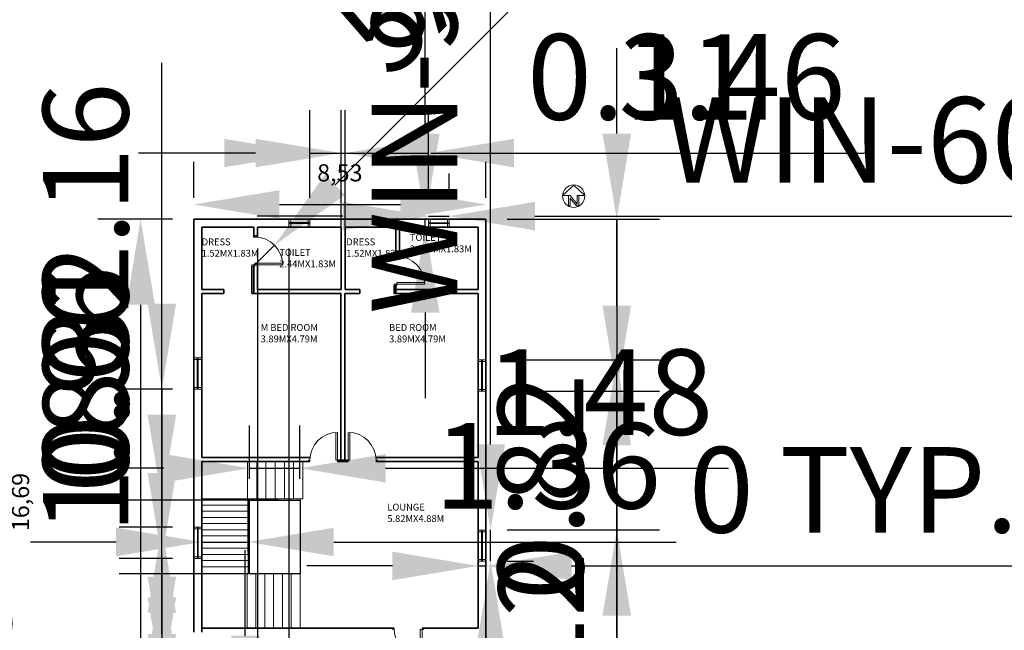
# Model space of a CAD drawing. Units: metres. Extents: x 1246 to 2549, y 2050 to 4184.
# Tile 4 of 6: x 1268 to 1297, y 2088 to 2106. Entities that reach past the tile are written whole.
import ezdxf

# ---------------------------------------------------------------- set-up
doc = ezdxf.new("R2010")
doc.units = ezdxf.units.M
for name, color, linetype, lineweight in [('A-ANNO-DIMS', 2, 'Continuous', 18), ('A-ANNO-SYMB', 7, 'Continuous', 18), ('A-AREA-IDEN', 7, 'Continuous', 18), ('A-DOOR', 3, 'Continuous', 18), ('A-FLOR-EVTR', 7, 'Continuous', 25), ('A-FLOR-STRS', 7, 'Continuous', 18), ('A-GLAZ', 4, 'Continuous', 18), ('A-WALL', 7, 'Continuous', 35)]:
    doc.layers.add(name, color=color, linetype=linetype, lineweight=lineweight)
doc.styles.get("Standard").update_dxf_attribs({"font": 'arial.ttf'})
doc.dimstyles.new('ISO-25', dxfattribs={"dimtxt": 2.5, "dimasz": 2.5, "dimexe": 1.25, "dimexo": 0.625, "dimtad": 1, "dimtxsty": 'Standard', "dimcen": 2.5, "dimadec": 0, "dimazin": 0, "dimtfac": 1, "dimtmove": 0, "dimatfit": 3, "dimfxl": 1, "dimarcsym": 0})

# ---------------------------------------------------------------- blocks, each defined once
blk = doc.blocks.new('*D1')
at = {"layer": 'A-ANNO-DIMS', "color": 0, "lineweight": -2, "transparency": 16777216}
for p, q in [((1273.334, 2100.834), (1273.334, 2101.888)), ((1281.867, 2100.834), (1281.867, 2101.888)), ((1275.834, 2100.638), (1279.367, 2100.638))]:
    blk.add_line(p, q, dxfattribs=at)
at = {"layer": 'A-ANNO-DIMS', "color": 0, "transparency": 16777216}
for points in [[(1275.834, 2101.055), (1275.834, 2100.221), (1273.334, 2100.638)], [(1279.367, 2101.055), (1279.367, 2100.221), (1281.867, 2100.638)]]:
    blk.add_solid(points, dxfattribs=at)
at = {"layer": 'Defpoints', "color": 0, "transparency": 16777216}
for p in [(1281.867, 2100.638), (1273.334, 2100.209), (1281.867, 2100.209)]:
    blk.add_point(p, dxfattribs=at)
at = {"layer": 'A-ANNO-DIMS', "color": 0, "transparency": 16777216, "insert": (1277.6, 2101.564), "char_height": 2.5, "attachment_point": 5}
blk.add_mtext('{\\H0.2x;8,53}', dxfattribs=at)
blk = doc.blocks.new('*D2')
at = {"layer": 'A-ANNO-DIMS', "color": 0, "lineweight": -2, "transparency": 16777216}
for p, q in [((1272.709, 2100.209), (1270.53, 2100.209)), ((1271.78, 2097.709), (1271.78, 2086.022)), ((1272.709, 2083.522), (1270.53, 2083.522))]:
    blk.add_line(p, q, dxfattribs=at)
at = {"layer": 'A-ANNO-DIMS', "color": 0, "transparency": 16777216}
for points in [[(1271.364, 2097.709), (1272.197, 2097.709), (1271.78, 2100.209)], [(1271.364, 2086.022), (1272.197, 2086.022), (1271.78, 2083.522)]]:
    blk.add_solid(points, dxfattribs=at)
at = {"layer": 'Defpoints', "color": 0, "transparency": 16777216}
for p in [(1273.334, 2100.209), (1271.78, 2083.522), (1273.334, 2083.522)]:
    blk.add_point(p, dxfattribs=at)
at = {"layer": 'A-ANNO-DIMS', "color": 0, "transparency": 16777216, "insert": (1264.522, 2091.865), "char_height": 2.5, "attachment_point": 5, "rotation": 90}
blk.add_mtext('{\\H0.4x;\\P\\H0.5x;\\P\\P\\P\\P\\P\\P\\P 16,69}', dxfattribs=at)
blk = doc.blocks.new('North Arrow')
for p, q in [((0, 0), (-12.86, -11.999)), ((0, 0), (12.782, -11.999)), ((-12.86, -11.999), (-6, -11.999)), ((-6, -11.999), (-6, -23.999)), ((-6, -11.999), (-4, -11.999)), ((-4, -11.999), (4, -21.999)), ((3.195, -23.996), (-4, -15.002)), ((-4, -15.002), (-4, -23.999)), ((4, -11.999), (4, -21.999)), ((6, -11.999), (4, -11.999)), ((12.782, -11.999), (6, -11.999)), ((6, -11.999), (6, -23.999)), ((-6, -23.999), (-4, -23.999)), ((6, -23.999), (3.195, -23.999))]:
    blk.add_line(p, q)
blk.add_circle((-0.013, -12.745), 12.885)
blk = doc.blocks.new('DOOR-SWING-813')
for p, q in [((0.033, 0.039), (0.033, 0.09)), ((0.033, 0.09), (0.844, 0.09))]:
    blk.add_line(p, q)
for points in [[(0.033, 0.852), (0.033, 0.891), (0.002, 0.891), (0.002, 0.852)], [(0.033, 0.039), (0.033, 0), (0, 0), (0, 0.039)]]:
    blk.add_lwpolyline(points, close=True)
blk.add_lwpolyline([(0.846, 0.039), (0.033, 0.039), (0.033, 0.09)])
blk.add_arc((0.033, 0.039), 0.813, 0, 90)
blk = doc.blocks.new('WIN-609')
for p, q in [((0, 0.23), (0.61, 0.23)), ((0, 0), (0, 0.23)), ((0, 0.128), (0.61, 0.128)), ((0, 0.115), (0.61, 0.115)), ((0, 0.102), (0.61, 0.102)), ((0.61, 0), (0, 0)), ((0, 0), (0.051, 0)), ((0.051, 0), (0.051, 0.23)), ((0.559, 0), (0.559, 0.23)), ((0.61, 0), (0.559, 0)), ((0.61, 0.23), (0.61, 0))]:
    blk.add_line(p, q)
blk = doc.blocks.new('WIN-914')
for p, q in [((0, 0), (0, 0.914)), ((0, 0.914), (0.23, 0.914)), ((0.23, 0.864), (0, 0.864)), ((0.102, 0), (0.102, 0.914)), ((0.115, 0), (0.115, 0.914)), ((0.128, 0), (0.128, 0.914)), ((0.23, 0.914), (0.23, 0)), ((0.23, 0.914), (0.23, 0.864)), ((0.23, 0.051), (0, 0.051)), ((0.23, 0), (0, 0)), ((0.23, 0), (0.23, 0.051))]:
    blk.add_line(p, q)
blk = doc.blocks.new('*D7')
at = {"layer": 'A-ANNO-DIMS', "color": 0, "lineweight": -2, "transparency": 16777216}
for p, q in [((1274.837, 2088.031), (1274.837, 2090.531)), ((1274.346, 2085.531), (1273.587, 2085.531)), ((1274.837, 2085.531), (1274.837, 2084.639)), ((1274.346, 2084.639), (1273.587, 2084.639)), ((1274.837, 2082.139), (1274.837, 2049.849))]:
    blk.add_line(p, q, dxfattribs=at)
at = {"layer": 'A-ANNO-DIMS', "color": 0, "transparency": 16777216}
for points in [[(1274.421, 2088.031), (1275.254, 2088.031), (1274.837, 2085.531)], [(1274.421, 2082.139), (1275.254, 2082.139), (1274.837, 2084.639)]]:
    blk.add_solid(points, dxfattribs=at)
at = {"layer": 'Defpoints', "color": 0, "transparency": 16777216}
for p in [(1274.971, 2085.531), (1274.837, 2084.639), (1274.971, 2084.639)]:
    blk.add_point(p, dxfattribs=at)
at = {"layer": 'A-ANNO-DIMS', "color": 0, "transparency": 16777216, "insert": (1272.918, 2064.744), "char_height": 2.5, "attachment_point": 5, "rotation": 90}
blk.add_mtext('DOOR-813 1 TYP.', dxfattribs=at)
blk = doc.blocks.new('*D8')
at = {"layer": 'A-ANNO-DIMS', "color": 0, "lineweight": -2, "transparency": 16777216}
for p, q in [((1274.971, 2086.156), (1274.971, 2086.914)), ((1275.817, 2086.156), (1275.817, 2086.914)), ((1272.471, 2085.664), (1258.73, 2085.664)), ((1275.817, 2085.664), (1274.971, 2085.664)), ((1278.317, 2085.664), (1280.817, 2085.664))]:
    blk.add_line(p, q, dxfattribs=at)
at = {"layer": 'A-ANNO-DIMS', "color": 0, "transparency": 16777216}
for points in [[(1272.471, 2086.081), (1272.471, 2085.248), (1274.971, 2085.664)], [(1278.317, 2086.081), (1278.317, 2085.248), (1275.817, 2085.664)]]:
    blk.add_solid(points, dxfattribs=at)
at = {"layer": 'Defpoints', "color": 0, "transparency": 16777216}
for p in [(1274.971, 2085.664), (1274.971, 2085.531), (1275.817, 2085.531)]:
    blk.add_point(p, dxfattribs=at)
at = {"layer": 'A-ANNO-DIMS', "color": 0, "transparency": 16777216, "insert": (1264.35, 2087.545), "char_height": 2.5, "attachment_point": 5}
blk.add_mtext('1 TYP.', dxfattribs=at)
blk = doc.blocks.new('*D9')
at = {"layer": 'A-ANNO-DIMS', "color": 0, "lineweight": -2, "transparency": 16777216}
for p, q in [((1282.004, 2093.624), (1282.004, 2122.452)), ((1282.004, 2090.21), (1282.004, 2091.124)), ((1282.492, 2091.124), (1283.254, 2091.124)), ((1282.492, 2090.21), (1283.254, 2090.21)), ((1282.004, 2087.71), (1282.004, 2085.21))]:
    blk.add_line(p, q, dxfattribs=at)
at = {"layer": 'A-ANNO-DIMS', "color": 0, "transparency": 16777216}
for points in [[(1281.587, 2093.624), (1282.42, 2093.624), (1282.004, 2091.124)], [(1281.587, 2087.71), (1282.42, 2087.71), (1282.004, 2090.21)]]:
    blk.add_solid(points, dxfattribs=at)
at = {"layer": 'Defpoints', "color": 0, "transparency": 16777216}
for p in [(1281.867, 2091.124), (1282.004, 2091.124), (1281.867, 2090.21)]:
    blk.add_point(p, dxfattribs=at)
at = {"layer": 'A-ANNO-DIMS', "color": 0, "transparency": 16777216, "insert": (1280.102, 2109.288), "char_height": 2.5, "attachment_point": 5, "rotation": 90}
blk.add_mtext('WIN-914 1 TYP.', dxfattribs=at)
blk = doc.blocks.new('*D10')
at = {"layer": 'A-ANNO-DIMS', "color": 0, "lineweight": -2, "transparency": 16777216}
for p, q in [((1279.137, 2090.073), (1276.637, 2090.073)), ((1281.637, 2090.073), (1281.867, 2090.073)), ((1284.367, 2090.073), (1298.343, 2090.073)), ((1281.637, 2089.585), (1281.637, 2088.823)), ((1281.867, 2089.585), (1281.867, 2088.823))]:
    blk.add_line(p, q, dxfattribs=at)
at = {"layer": 'A-ANNO-DIMS', "color": 0, "transparency": 16777216}
for points in [[(1279.137, 2090.489), (1279.137, 2089.656), (1281.637, 2090.073)], [(1284.367, 2090.489), (1284.367, 2089.656), (1281.867, 2090.073)]]:
    blk.add_solid(points, dxfattribs=at)
at = {"layer": 'Defpoints', "color": 0, "transparency": 16777216}
for p in [(1281.637, 2090.21), (1281.867, 2090.21), (1281.867, 2090.073)]:
    blk.add_point(p, dxfattribs=at)
at = {"layer": 'A-ANNO-DIMS', "color": 0, "transparency": 16777216, "insert": (1292.605, 2091.974), "char_height": 2.5, "attachment_point": 5}
blk.add_mtext('0 TYP.', dxfattribs=at)
blk = doc.blocks.new('*D11')
at = {"layer": 'A-ANNO-DIMS', "color": 0, "lineweight": -2, "transparency": 16777216}
for p, q in [((1280.187, 2100.832), (1280.187, 2101.548)), ((1280.797, 2100.832), (1280.797, 2101.548)), ((1277.687, 2100.298), (1275.187, 2100.298)), ((1280.187, 2100.298), (1280.797, 2100.298)), ((1283.297, 2100.298), (1312.125, 2100.298))]:
    blk.add_line(p, q, dxfattribs=at)
at = {"layer": 'A-ANNO-DIMS', "color": 0, "transparency": 16777216}
for points in [[(1277.687, 2100.715), (1277.687, 2099.882), (1280.187, 2100.298)], [(1283.297, 2100.715), (1283.297, 2099.882), (1280.797, 2100.298)]]:
    blk.add_solid(points, dxfattribs=at)
at = {"layer": 'Defpoints', "color": 0, "transparency": 16777216}
for p in [(1280.187, 2100.207), (1280.797, 2100.298), (1280.797, 2100.207)]:
    blk.add_point(p, dxfattribs=at)
at = {"layer": 'A-ANNO-DIMS', "color": 0, "transparency": 16777216, "insert": (1298.961, 2102.2), "char_height": 2.5, "attachment_point": 5}
blk.add_mtext('WIN-609 1 TYP.', dxfattribs=at)
blk = doc.blocks.new('*D12')
at = {"layer": 'A-ANNO-DIMS', "color": 0, "lineweight": -2, "transparency": 16777216}
for p, q in [((1280.096, 2102.707), (1280.096, 2116.684)), ((1279.562, 2100.207), (1278.846, 2100.207)), ((1280.096, 2099.977), (1280.096, 2100.207)), ((1279.562, 2099.977), (1278.846, 2099.977)), ((1280.096, 2097.477), (1280.096, 2094.977))]:
    blk.add_line(p, q, dxfattribs=at)
at = {"layer": 'A-ANNO-DIMS', "color": 0, "transparency": 16777216}
for points in [[(1279.679, 2102.707), (1280.513, 2102.707), (1280.096, 2100.207)], [(1279.679, 2097.477), (1280.513, 2097.477), (1280.096, 2099.977)]]:
    blk.add_solid(points, dxfattribs=at)
at = {"layer": 'Defpoints', "color": 0, "transparency": 16777216}
for p in [(1280.096, 2100.207), (1280.187, 2100.207), (1280.187, 2099.977)]:
    blk.add_point(p, dxfattribs=at)
at = {"layer": 'A-ANNO-DIMS', "color": 0, "transparency": 16777216, "insert": (1278.195, 2110.945), "char_height": 2.5, "attachment_point": 5, "rotation": 90}
blk.add_mtext('0 TYP.', dxfattribs=at)
blk = doc.blocks.new('*D14')
at = {"layer": 'A-ANNO-DIMS', "color": 0, "lineweight": -2, "transparency": 16777216}
for p, q in [((1285.689, 2086.022), (1285.689, 2096.24)), ((1282.492, 2083.522), (1286.939, 2083.522)), ((1285.689, 2082.699), (1285.689, 2083.522)), ((1282.492, 2082.699), (1286.939, 2082.699)), ((1285.689, 2080.199), (1285.689, 2077.699))]:
    blk.add_line(p, q, dxfattribs=at)
at = {"layer": 'A-ANNO-DIMS', "color": 0, "transparency": 16777216}
for points in [[(1285.272, 2086.022), (1286.106, 2086.022), (1285.689, 2083.522)], [(1285.272, 2080.199), (1286.106, 2080.199), (1285.689, 2082.699)]]:
    blk.add_solid(points, dxfattribs=at)
at = {"layer": 'Defpoints', "color": 0, "transparency": 16777216}
for p in [(1281.867, 2083.522), (1285.689, 2083.522), (1281.867, 2082.699)]:
    blk.add_point(p, dxfattribs=at)
at = {"layer": 'A-ANNO-DIMS', "color": 0, "transparency": 16777216, "insert": (1283.788, 2092.381), "char_height": 2.5, "attachment_point": 5, "rotation": 90}
blk.add_mtext('0.82', dxfattribs=at)
blk = doc.blocks.new('*D15')
at = {"layer": 'A-ANNO-DIMS', "color": 0, "lineweight": -2, "transparency": 16777216}
for p, q in [((1272.401, 2088.082), (1272.401, 2098.09)), ((1272.939, 2085.582), (1271.151, 2085.582)), ((1272.401, 2083.752), (1272.401, 2085.582)), ((1272.939, 2083.752), (1271.151, 2083.752)), ((1272.401, 2081.252), (1272.401, 2078.752))]:
    blk.add_line(p, q, dxfattribs=at)
at = {"layer": 'A-ANNO-DIMS', "color": 0, "transparency": 16777216}
for points in [[(1271.985, 2088.082), (1272.818, 2088.082), (1272.401, 2085.582)], [(1271.985, 2081.252), (1272.818, 2081.252), (1272.401, 2083.752)]]:
    blk.add_solid(points, dxfattribs=at)
at = {"layer": 'Defpoints', "color": 0, "transparency": 16777216}
for p in [(1272.401, 2085.582), (1273.564, 2085.582), (1273.564, 2083.752)]:
    blk.add_point(p, dxfattribs=at)
at = {"layer": 'A-ANNO-DIMS', "color": 0, "transparency": 16777216, "insert": (1270.499, 2094.336), "char_height": 2.5, "attachment_point": 5, "rotation": 90}
blk.add_mtext('1.83', dxfattribs=at)
blk = doc.blocks.new('*D17')
at = {"layer": 'A-ANNO-DIMS', "color": 0, "lineweight": -2, "transparency": 16777216}
for p, q in [((1275.198, 2099.354), (1275.198, 2080.517)), ((1276.114, 2099.356), (1276.114, 2080.517)), ((1272.698, 2081.767), (1270.198, 2081.767)), ((1275.198, 2081.767), (1276.114, 2081.767)), ((1278.614, 2081.767), (1288.832, 2081.767))]:
    blk.add_line(p, q, dxfattribs=at)
at = {"layer": 'A-ANNO-DIMS', "color": 0, "transparency": 16777216}
for points in [[(1272.698, 2082.183), (1272.698, 2081.35), (1275.198, 2081.767)], [(1278.614, 2082.183), (1278.614, 2081.35), (1276.114, 2081.767)]]:
    blk.add_solid(points, dxfattribs=at)
at = {"layer": 'Defpoints', "color": 0, "transparency": 16777216}
for p in [(1275.198, 2099.979), (1276.114, 2099.981), (1276.114, 2081.767)]:
    blk.add_point(p, dxfattribs=at)
at = {"layer": 'A-ANNO-DIMS', "color": 0, "transparency": 16777216, "insert": (1284.973, 2083.668), "char_height": 2.5, "attachment_point": 5}
blk.add_mtext('0.92', dxfattribs=at)
blk = doc.blocks.new('*D18')
at = {"layer": 'A-ANNO-DIMS', "color": 0, "lineweight": -2, "transparency": 16777216}
for p, q in [((1276.723, 2100.836), (1276.723, 2103.391)), ((1280.187, 2100.832), (1280.187, 2103.391)), ((1274.223, 2102.141), (1271.723, 2102.141)), ((1276.723, 2102.141), (1280.187, 2102.141)), ((1282.687, 2102.141), (1292.928, 2102.141))]:
    blk.add_line(p, q, dxfattribs=at)
at = {"layer": 'A-ANNO-DIMS', "color": 0, "transparency": 16777216}
for points in [[(1274.223, 2102.558), (1274.223, 2101.725), (1276.723, 2102.141)], [(1282.687, 2102.558), (1282.687, 2101.725), (1280.187, 2102.141)]]:
    blk.add_solid(points, dxfattribs=at)
at = {"layer": 'Defpoints', "color": 0, "transparency": 16777216}
for p in [(1280.187, 2102.141), (1276.723, 2100.211), (1280.187, 2100.207)]:
    blk.add_point(p, dxfattribs=at)
at = {"layer": 'A-ANNO-DIMS', "color": 0, "transparency": 16777216, "insert": (1289.058, 2104.044), "char_height": 2.5, "attachment_point": 5}
blk.add_mtext('3.46', dxfattribs=at)
blk = doc.blocks.new('*D19')
at = {"layer": 'A-ANNO-DIMS', "color": 0, "lineweight": -2, "transparency": 16777216}
for p, q in [((1285.689, 2102.709), (1285.689, 2105.209)), ((1282.492, 2100.209), (1286.939, 2100.209)), ((1285.689, 2100.209), (1285.689, 2096.096)), ((1282.492, 2096.096), (1286.939, 2096.096)), ((1285.689, 2093.596), (1285.689, 2081.335))]:
    blk.add_line(p, q, dxfattribs=at)
at = {"layer": 'A-ANNO-DIMS', "color": 0, "transparency": 16777216}
for points in [[(1285.272, 2102.709), (1286.106, 2102.709), (1285.689, 2100.209)], [(1285.272, 2093.596), (1286.106, 2093.596), (1285.689, 2096.096)]]:
    blk.add_solid(points, dxfattribs=at)
at = {"layer": 'Defpoints', "color": 0, "transparency": 16777216}
for p in [(1281.867, 2100.209), (1281.867, 2096.096), (1285.689, 2096.096)]:
    blk.add_point(p, dxfattribs=at)
at = {"layer": 'A-ANNO-DIMS', "color": 0, "transparency": 16777216, "insert": (1283.809, 2086.216), "char_height": 2.5, "attachment_point": 5, "rotation": 90}
blk.add_mtext('4.112', dxfattribs=at)
blk = doc.blocks.new('*D20')
at = {"layer": 'A-ANNO-DIMS', "color": 0, "lineweight": -2, "transparency": 16777216}
for p, q in [((1285.689, 2097.682), (1285.689, 2100.182)), ((1282.492, 2095.182), (1286.939, 2095.182)), ((1285.689, 2095.182), (1285.689, 2091.124)), ((1282.492, 2091.124), (1286.939, 2091.124)), ((1285.689, 2088.624), (1285.689, 2078.281))]:
    blk.add_line(p, q, dxfattribs=at)
at = {"layer": 'A-ANNO-DIMS', "color": 0, "transparency": 16777216}
for points in [[(1285.272, 2097.682), (1286.106, 2097.682), (1285.689, 2095.182)], [(1285.272, 2088.624), (1286.106, 2088.624), (1285.689, 2091.124)]]:
    blk.add_solid(points, dxfattribs=at)
at = {"layer": 'Defpoints', "color": 0, "transparency": 16777216}
for p in [(1281.867, 2095.182), (1281.867, 2091.124), (1285.689, 2091.124)]:
    blk.add_point(p, dxfattribs=at)
at = {"layer": 'A-ANNO-DIMS', "color": 0, "transparency": 16777216, "insert": (1283.788, 2082.203), "char_height": 2.5, "attachment_point": 5, "rotation": 90}
blk.add_mtext('4.06', dxfattribs=at)
blk = doc.blocks.new('*D21')
at = {"layer": 'A-ANNO-DIMS', "color": 0, "lineweight": -2, "transparency": 16777216}
for p, q in [((1272.401, 2097.74), (1272.401, 2100.24)), ((1272.709, 2095.24), (1271.151, 2095.24)), ((1272.401, 2095.24), (1272.401, 2091.205)), ((1272.711, 2091.205), (1271.151, 2091.205)), ((1272.401, 2088.705), (1272.401, 2076.429))]:
    blk.add_line(p, q, dxfattribs=at)
at = {"layer": 'A-ANNO-DIMS', "color": 0, "transparency": 16777216}
for points in [[(1271.985, 2097.74), (1272.818, 2097.74), (1272.401, 2095.24)], [(1271.985, 2088.705), (1272.818, 2088.705), (1272.401, 2091.205)]]:
    blk.add_solid(points, dxfattribs=at)
at = {"layer": 'Defpoints', "color": 0, "transparency": 16777216}
for p in [(1273.334, 2095.24), (1272.401, 2091.205), (1273.336, 2091.205)]:
    blk.add_point(p, dxfattribs=at)
at = {"layer": 'A-ANNO-DIMS', "color": 0, "transparency": 16777216, "insert": (1270.499, 2081.317), "char_height": 2.5, "attachment_point": 5, "rotation": 90}
blk.add_mtext('4.034', dxfattribs=at)
blk = doc.blocks.new('*D22')
at = {"layer": 'A-ANNO-DIMS', "color": 0, "lineweight": -2, "transparency": 16777216}
for p, q in [((1272.401, 2092.791), (1272.401, 2095.291)), ((1272.711, 2090.291), (1271.151, 2090.291)), ((1272.401, 2090.291), (1272.401, 2087.264)), ((1272.708, 2087.264), (1271.151, 2087.264)), ((1272.401, 2084.764), (1272.401, 2074.522))]:
    blk.add_line(p, q, dxfattribs=at)
at = {"layer": 'A-ANNO-DIMS', "color": 0, "transparency": 16777216}
for points in [[(1271.985, 2092.791), (1272.818, 2092.791), (1272.401, 2090.291)], [(1271.985, 2084.764), (1272.818, 2084.764), (1272.401, 2087.264)]]:
    blk.add_solid(points, dxfattribs=at)
at = {"layer": 'Defpoints', "color": 0, "transparency": 16777216}
for p in [(1273.336, 2090.291), (1272.401, 2087.264), (1273.333, 2087.264)]:
    blk.add_point(p, dxfattribs=at)
at = {"layer": 'A-ANNO-DIMS', "color": 0, "transparency": 16777216, "insert": (1270.499, 2078.393), "char_height": 2.5, "attachment_point": 5, "rotation": 90}
blk.add_mtext('3.03', dxfattribs=at)
blk = doc.blocks.new('*D23')
at = {"layer": 'A-ANNO-DIMS', "color": 0, "lineweight": -2, "transparency": 16777216}
for p, q in [((1273.564, 2090.465), (1273.564, 2092.022)), ((1274.92, 2090.465), (1274.92, 2092.022)), ((1271.064, 2090.772), (1268.564, 2090.772)), ((1273.564, 2090.772), (1274.92, 2090.772)), ((1277.42, 2090.772), (1287.426, 2090.772))]:
    blk.add_line(p, q, dxfattribs=at)
at = {"layer": 'A-ANNO-DIMS', "color": 0, "transparency": 16777216}
for points in [[(1271.064, 2091.189), (1271.064, 2090.356), (1273.564, 2090.772)], [(1277.42, 2091.189), (1277.42, 2090.356), (1274.92, 2090.772)]]:
    blk.add_solid(points, dxfattribs=at)
at = {"layer": 'Defpoints', "color": 0, "transparency": 16777216}
for p in [(1274.92, 2090.772), (1273.564, 2089.84), (1274.92, 2089.84)]:
    blk.add_point(p, dxfattribs=at)
at = {"layer": 'A-ANNO-DIMS', "color": 0, "transparency": 16777216, "insert": (1283.673, 2092.675), "char_height": 2.5, "attachment_point": 5}
blk.add_mtext('1.36', dxfattribs=at)
blk = doc.blocks.new('*D24')
at = {"layer": 'A-ANNO-DIMS', "color": 0, "lineweight": -2, "transparency": 16777216}
for p, q in [((1274.96, 2092.622), (1274.96, 2094.179)), ((1276.436, 2092.622), (1276.436, 2094.179)), ((1272.46, 2092.929), (1269.96, 2092.929)), ((1274.96, 2092.929), (1276.436, 2092.929)), ((1278.936, 2092.929), (1288.95, 2092.929))]:
    blk.add_line(p, q, dxfattribs=at)
at = {"layer": 'A-ANNO-DIMS', "color": 0, "transparency": 16777216}
for points in [[(1272.46, 2093.345), (1272.46, 2092.512), (1274.96, 2092.929)], [(1278.936, 2093.345), (1278.936, 2092.512), (1276.436, 2092.929)]]:
    blk.add_solid(points, dxfattribs=at)
at = {"layer": 'Defpoints', "color": 0, "transparency": 16777216}
for p in [(1276.436, 2092.929), (1274.96, 2091.997), (1276.436, 2091.997)]:
    blk.add_point(p, dxfattribs=at)
at = {"layer": 'A-ANNO-DIMS', "color": 0, "transparency": 16777216, "insert": (1285.193, 2094.83), "char_height": 2.5, "attachment_point": 5}
blk.add_mtext('1.48', dxfattribs=at)
blk = doc.blocks.new('*D25')
at = {"layer": 'A-ANNO-DIMS', "color": 0, "lineweight": -2, "transparency": 16777216}
for p, q in [((1272.401, 2094.497), (1272.401, 2104.781)), ((1275.811, 2091.997), (1271.151, 2091.997)), ((1272.401, 2089.84), (1272.401, 2091.997)), ((1275.811, 2089.84), (1271.151, 2089.84)), ((1272.401, 2087.34), (1272.401, 2084.84))]:
    blk.add_line(p, q, dxfattribs=at)
at = {"layer": 'A-ANNO-DIMS', "color": 0, "transparency": 16777216}
for points in [[(1271.985, 2094.497), (1272.818, 2094.497), (1272.401, 2091.997)], [(1271.985, 2087.34), (1272.818, 2087.34), (1272.401, 2089.84)]]:
    blk.add_solid(points, dxfattribs=at)
at = {"layer": 'Defpoints', "color": 0, "transparency": 16777216}
for p in [(1272.401, 2091.997), (1276.436, 2091.997), (1276.436, 2089.84)]:
    blk.add_point(p, dxfattribs=at)
at = {"layer": 'A-ANNO-DIMS', "color": 0, "transparency": 16777216, "insert": (1270.5, 2100.889), "char_height": 2.5, "attachment_point": 5, "rotation": 90}
blk.add_mtext('2.16', dxfattribs=at)
blk = doc.blocks.new('*D27')
at = {"layer": 'A-ANNO-DIMS', "color": 0, "lineweight": -2, "transparency": 16777216}
for p, q in [((1277.638, 2098.774), (1277.638, 2103.391)), ((1277.753, 2098.774), (1277.753, 2103.391)), ((1275.138, 2102.141), (1272.638, 2102.141)), ((1277.638, 2102.141), (1277.753, 2102.141)), ((1280.253, 2102.141), (1290.014, 2102.141))]:
    blk.add_line(p, q, dxfattribs=at)
at = {"layer": 'A-ANNO-DIMS', "color": 0, "transparency": 16777216}
for points in [[(1275.138, 2102.558), (1275.138, 2101.725), (1277.638, 2102.141)], [(1280.253, 2102.558), (1280.253, 2101.725), (1277.753, 2102.141)]]:
    blk.add_solid(points, dxfattribs=at)
at = {"layer": 'Defpoints', "color": 0, "transparency": 16777216}
for p in [(1277.753, 2102.141), (1277.638, 2098.149), (1277.753, 2098.149)]:
    blk.add_point(p, dxfattribs=at)
at = {"layer": 'A-ANNO-DIMS', "color": 0, "transparency": 16777216, "insert": (1286.383, 2104.043), "char_height": 2.5, "attachment_point": 5}
blk.add_mtext('0.11', dxfattribs=at)
blk = doc.blocks.new('*D28')
at = {"layer": 'A-ANNO-DIMS', "color": 0, "lineweight": -2, "transparency": 16777216}
for p, q in [((1272.401, 2089.155), (1272.401, 2099.397)), ((1272.938, 2086.655), (1271.151, 2086.655)), ((1272.401, 2085.696), (1272.401, 2086.655)), ((1272.939, 2085.696), (1271.151, 2085.696)), ((1272.401, 2083.196), (1272.401, 2080.696))]:
    blk.add_line(p, q, dxfattribs=at)
at = {"layer": 'A-ANNO-DIMS', "color": 0, "transparency": 16777216}
for points in [[(1271.985, 2089.155), (1272.818, 2089.155), (1272.401, 2086.655)], [(1271.985, 2083.196), (1272.818, 2083.196), (1272.401, 2085.696)]]:
    blk.add_solid(points, dxfattribs=at)
at = {"layer": 'Defpoints', "color": 0, "transparency": 16777216}
for p in [(1272.401, 2086.655), (1273.563, 2086.655), (1273.564, 2085.696)]:
    blk.add_point(p, dxfattribs=at)
at = {"layer": 'A-ANNO-DIMS', "color": 0, "transparency": 16777216, "insert": (1270.5, 2095.526), "char_height": 2.5, "attachment_point": 5, "rotation": 90}
blk.add_mtext('0.96', dxfattribs=at)
blk = doc.blocks.new('*D29')
at = {"layer": 'A-ANNO-DIMS', "color": 0, "lineweight": -2, "transparency": 16777216}
for p, q in [((1272.401, 2089.764), (1272.401, 2099.525)), ((1272.708, 2087.264), (1271.151, 2087.264)), ((1272.401, 2086.655), (1272.401, 2087.264)), ((1272.708, 2086.655), (1271.151, 2086.655)), ((1272.401, 2084.155), (1272.401, 2081.655))]:
    blk.add_line(p, q, dxfattribs=at)
at = {"layer": 'A-ANNO-DIMS', "color": 0, "transparency": 16777216}
for points in [[(1271.985, 2089.764), (1272.818, 2089.764), (1272.401, 2087.264)], [(1271.985, 2084.155), (1272.818, 2084.155), (1272.401, 2086.655)]]:
    blk.add_solid(points, dxfattribs=at)
at = {"layer": 'Defpoints', "color": 0, "transparency": 16777216}
for p in [(1272.401, 2087.264), (1273.333, 2087.264), (1273.333, 2086.655)]:
    blk.add_point(p, dxfattribs=at)
at = {"layer": 'A-ANNO-DIMS', "color": 0, "transparency": 16777216, "insert": (1270.5, 2095.894), "char_height": 2.5, "attachment_point": 5, "rotation": 90}
blk.add_mtext('0.61', dxfattribs=at)
blk = doc.blocks.new('*D30')
at = {"layer": 'A-ANNO-DIMS', "color": 0, "lineweight": -2, "transparency": 16777216}
for p, q in [((1289.848, 2113.612), (1277.459, 2101.216)), ((1275.117, 2098.873), (1275.692, 2099.448))]:
    blk.add_line(p, q, dxfattribs=at)
at = {"layer": 'A-ANNO-DIMS', "color": 0, "transparency": 16777216}
blk.add_solid([(1277.164, 2101.511), (1277.754, 2100.921), (1275.692, 2099.448)], dxfattribs=at)
at = {"layer": 'Defpoints', "color": 0, "transparency": 16777216}
for p in [(1275.692, 2099.448), (1275.117, 2098.873)]:
    blk.add_point(p, dxfattribs=at)
at = {"layer": 'A-ANNO-DIMS', "color": 0, "transparency": 16777216, "insert": (1283.192, 2109.642), "char_height": 2.5, "attachment_point": 5, "rotation": 45.0176}
blk.add_mtext('5X R0.81', dxfattribs=at)

msp = doc.modelspace()

# ---------------------------------------------------------------- linework, layer by layer
at = {"layer": 'A-DOOR'}
for p, q in [((1275.0332, 2098.8342), (1275.0332, 2098.8728)), ((1275.0332, 2098.8728), (1275.084, 2098.8728)), ((1279.1818, 2098.2722), (1279.1818, 2098.3108)), ((1279.1818, 2098.3108), (1279.2326, 2098.3108))]:
    msp.add_line(p, q, dxfattribs=at)
at = {"layer": 'A-FLOR-EVTR'}
msp.add_lwpolyline([(1274.9599, 2091.9965), (1276.4362, 2091.9965), (1276.4362, 2089.8402), (1274.9599, 2089.8402)], close=True, dxfattribs=at)
at = {"layer": 'A-FLOR-STRS'}
for p, q in [((1274.9017, 2092.0333), (1274.9017, 2093.1302)), ((1275.1711, 2092.0333), (1275.1711, 2093.1302)), ((1275.4405, 2092.0333), (1275.4405, 2093.1302)), ((1275.7099, 2092.0333), (1275.7099, 2093.1302)), ((1275.9793, 2092.0333), (1275.9793, 2093.1302)), ((1276.2488, 2092.0333), (1276.2488, 2093.1302)), ((1276.5182, 2093.1302), (1276.5182, 2092.0333)), ((1276.5182, 2092.0333), (1276.5182, 2093.1302)), ((1274.9196, 2092.0333), (1273.564, 2092.0333)), ((1274.9196, 2091.8529), (1273.564, 2091.8529)), ((1276.5182, 2092.0333), (1274.9196, 2092.0333)), ((1274.9196, 2092.0333), (1274.9196, 2089.8402)), ((1276.4362, 2089.8402), (1276.4362, 2092.0333)), ((1274.9196, 2091.6726), (1273.564, 2091.6726)), ((1274.9196, 2091.4922), (1273.564, 2091.4922)), ((1274.9196, 2091.3119), (1273.564, 2091.3119)), ((1274.9196, 2091.1316), (1273.564, 2091.1316)), ((1274.9196, 2090.9512), (1273.564, 2090.9512)), ((1274.9196, 2090.7709), (1273.564, 2090.7709)), ((1274.9196, 2090.5905), (1273.564, 2090.5905)), ((1274.9196, 2090.4102), (1273.564, 2090.4102)), ((1274.9196, 2090.2299), (1273.564, 2090.2299)), ((1274.9196, 2090.0495), (1273.564, 2090.0495)), ((1274.9196, 2089.8402), (1273.564, 2089.8402)), ((1273.564, 2089.8402), (1273.564, 2089.8402)), ((1274.8914, 2089.8402), (1274.8914, 2088.2502)), ((1274.9196, 2089.8402), (1276.4362, 2089.8402)), ((1275.1488, 2089.8402), (1275.1488, 2088.2502)), ((1275.4063, 2089.8402), (1275.4063, 2088.2502)), ((1275.6638, 2089.8402), (1275.6638, 2088.2502)), ((1275.9212, 2089.8402), (1275.9212, 2088.2502)), ((1276.1787, 2089.8402), (1276.1787, 2088.2502)), ((1276.4362, 2089.8402), (1276.4362, 2088.2502)), ((1276.4362, 2089.8402), (1276.4362, 2088.2502))]:
    msp.add_line(p, q, dxfattribs=at)
at = {"layer": 'A-WALL'}
for p, q in [((1273.334, 2098.1488), (1273.334, 2100.2088)), ((1273.334, 2100.2088), (1275.084, 2100.2088)), ((1275.084, 2100.2088), (1277.7526, 2100.2088)), ((1277.7526, 2100.2088), (1279.2326, 2100.2088)), ((1279.2326, 2100.2088), (1281.8669, 2100.2088)), ((1281.8669, 2100.2088), (1281.8669, 2098.1488)), ((1273.564, 2099.9788), (1275.084, 2099.9788)), ((1273.564, 2098.1488), (1273.564, 2099.9788)), ((1275.084, 2099.9788), (1275.084, 2099.6849)), ((1275.1983, 2099.9788), (1275.1983, 2099.6815)), ((1275.1983, 2099.9788), (1277.6383, 2099.9788)), ((1277.6383, 2099.9788), (1277.6383, 2098.1488)), ((1277.7526, 2099.9788), (1277.7526, 2098.1488)), ((1277.7526, 2099.9788), (1279.2326, 2099.9788)), ((1279.2326, 2099.9788), (1279.2326, 2099.1229)), ((1279.3469, 2099.9788), (1279.3469, 2099.1195)), ((1279.3469, 2099.9788), (1281.6369, 2099.9788)), ((1281.6369, 2099.9788), (1281.6369, 2098.1488)), ((1275.084, 2099.7255), (1275.1983, 2099.7255)), ((1279.2343, 2099.1635), (1279.3469, 2099.1635)), ((1275.0332, 2098.0345), (1275.0332, 2098.8342)), ((1275.084, 2098.8728), (1275.084, 2098.1488)), ((1275.1983, 2098.9236), (1275.1983, 2098.1488)), ((1273.334, 2098.1488), (1273.334, 2093.2445)), ((1274.2107, 2098.1488), (1273.564, 2098.1488)), ((1274.0223, 2098.1488), (1274.2107, 2098.1488)), ((1274.2107, 2098.1488), (1274.2107, 2098.0345)), ((1275.084, 2098.1488), (1275.084, 2098.0345)), ((1277.6383, 2098.1488), (1275.1983, 2098.1488)), ((1277.7526, 2098.1488), (1277.9598, 2098.1488)), ((1277.9598, 2098.1488), (1278.1807, 2098.1488)), ((1278.1807, 2098.1488), (1278.1807, 2098.0345)), ((1279.1818, 2098.0345), (1279.1818, 2098.2722)), ((1279.2326, 2098.1488), (1279.1818, 2098.1488)), ((1279.1818, 2098.1488), (1281.6369, 2098.1488)), ((1279.2326, 2098.3108), (1279.2326, 2098.1488)), ((1279.2326, 2098.1488), (1279.2326, 2098.0345)), ((1281.6369, 2098.1488), (1279.3469, 2098.1488)), ((1281.8669, 2098.1488), (1281.8669, 2093.1302)), ((1273.564, 2098.0345), (1273.564, 2093.2445)), ((1274.2107, 2098.0345), (1273.564, 2098.0345)), ((1275.084, 2098.0345), (1275.0332, 2098.0345)), ((1275.084, 2098.0345), (1275.0332, 2098.0345)), ((1277.6383, 2098.0345), (1275.084, 2098.0345)), ((1277.6326, 2093.2445), (1277.6326, 2098.0345)), ((1277.7469, 2093.2445), (1277.7469, 2098.0345)), ((1277.7469, 2093.2445), (1277.7469, 2098.0345)), ((1277.9598, 2098.0345), (1277.7469, 2098.0345)), ((1278.1807, 2098.0345), (1277.9598, 2098.0345)), ((1279.2326, 2098.0345), (1279.1818, 2098.0345)), ((1279.2326, 2098.0345), (1279.1818, 2098.0345)), ((1279.2326, 2098.0345), (1279.1818, 2098.0345)), ((1279.1818, 2098.0345), (1281.6369, 2098.0345)), ((1281.6369, 2098.0345), (1279.3469, 2098.0345)), ((1281.6369, 2098.0345), (1281.6369, 2093.2445)), ((1273.334, 2093.2445), (1273.334, 2088.1359)), ((1273.564, 2093.2445), (1276.7274, 2093.2445)), ((1275.8169, 2093.2445), (1276.7274, 2093.2445)), ((1277.6326, 2093.2445), (1277.6326, 2093.1302)), ((1277.7469, 2093.2445), (1277.7469, 2093.1302)), ((1281.6369, 2093.2445), (1278.6522, 2093.2445)), ((1273.564, 2093.1302), (1276.724, 2093.1302)), ((1273.564, 2093.1302), (1273.564, 2088.1359)), ((1273.564, 2093.1302), (1275.7026, 2093.1302)), ((1275.8169, 2093.1302), (1276.724, 2093.1302)), ((1276.6834, 2093.1302), (1276.5182, 2093.1302)), ((1276.724, 2093.1302), (1276.6834, 2093.1302)), ((1277.5361, 2093.1302), (1277.644, 2093.1302)), ((1277.5361, 2093.1302), (1277.8435, 2093.1302)), ((1277.5746, 2093.1633), (1277.8049, 2093.1633)), ((1277.6326, 2093.1302), (1277.5746, 2093.1302)), ((1277.7469, 2093.1302), (1277.8049, 2093.1302)), ((1277.8435, 2093.1302), (1277.7469, 2093.1302)), ((1281.6369, 2093.1302), (1278.6556, 2093.1302)), ((1278.6556, 2093.1302), (1281.6369, 2093.1302)), ((1281.6369, 2093.1302), (1281.6369, 2088.2502)), ((1281.8669, 2093.1302), (1281.8669, 2088.2502)), ((1281.8669, 2087.9121), (1281.8669, 2088.4556)), ((1273.564, 2088.2502), (1275.8169, 2088.2502)), ((1279.1883, 2088.2502), (1275.8169, 2088.2502)), ((1281.6369, 2088.2502), (1280.0004, 2088.2502)), ((1280.0969, 2088.2502), (1280.0389, 2088.2502)), ((1280.0969, 2088.2502), (1280.0969, 2088.2502))]:
    msp.add_line(p, q, dxfattribs=at)

# ---------------------------------------------------------------- block references
at = {"layer": 'A-ANNO-SYMB', "xscale": 0.0254, "yscale": 0.0254, "zscale": 0.0254}
msp.add_blockref('North Arrow', (1284.4301, 2101.2059), dxfattribs=at)
at = {"layer": 'A-DOOR'}
for p in [(1275.084, 2098.834), (1279.2326, 2098.272)]:
    msp.add_blockref('DOOR-SWING-813', p, dxfattribs=at)
at = {"layer": 'A-DOOR', "rotation": 90.00000000008399}
msp.add_blockref('DOOR-SWING-813', (1277.5749, 2093.1301), dxfattribs=at)
at = {"layer": 'A-DOOR', "extrusion": (0, 0, -1), "zscale": -1}
for p, rotation in [((-1277.8047, 2093.1301), 90.00000000008399), ((-1280.0392, 2088.2502), 270.0000000000915)]:
    msp.add_blockref('DOOR-SWING-813', p, dxfattribs=dict(at, rotation=rotation))
at = {"layer": 'A-GLAZ'}
for name, p in [('WIN-609', (1276.1134, 2099.981)), ('WIN-609', (1280.187, 2099.977)), ('WIN-914', (1273.3341, 2095.2392)), ('WIN-914', (1281.637, 2095.182)), ('WIN-914', (1273.3358, 2090.2909)), ('WIN-914', (1281.6367, 2090.2095))]:
    msp.add_blockref(name, p, dxfattribs=at)

# ---------------------------------------------------------------- texts
at = {"layer": 'A-AREA-IDEN', "attachment_point": 1}
for s, width, insert, char_height in [('\\P\\P\\P\\P\\P{\\H1.6x;\\P\\P\\P\\P\\P\\P\\P\\P\\P\\P\\P\\P\\P\\P\\P\\P\\P\\PDREESS }', 2.024418, (1273.4284, 2100.4903), 0.005), ('{\\H0.4x;\\PDRESS\\P1.52MX1.83M}', 2.167266, (1273.564, 2099.9788), 0.5), ('{\\H0.4x;\\PDRESS\\P1.52MX1.83M}', 2.167266, (1277.7877, 2099.9788), 0.5), ('{\\H0.4x;TOILET\\P2.289MX1.83M}', 2.167266, (1279.6449, 2099.7747), 0.5), ('{\\H0.4x;TOILET\\P2.44MX1.83M}', 2.167266, (1275.8309, 2099.3375), 0.5), ('{\\H0.4x;M BED ROOM\\P3.89MX4.79M}', 2.167266, (1275.2875, 2097.1436), 0.5), ('{\\H0.4x;BED ROOM\\P3.89MX4.79M}', 2.167266, (1279.0387, 2097.1436), 0.5), ('{\\H0.4x;LOUNGE\\P5.82MX4.88M}', 2.167266, (1278.9873, 2091.8917), 0.5)]:
    msp.add_mtext_dynamic_manual_height_columns(s, width=width, gutter_width=12.5, heights=[0], dxfattribs=dict(at, insert=insert, char_height=char_height))

# ---------------------------------------------------------------- dimensions: what is measured, and where the dimension line sits
at = {"layer": 'A-ANNO-DIMS'}
for base, p1, p2, angle, text, override, picture, middle in [((1282.0037, 2091.1239), (1281.8666, 2090.2099), (1281.8666, 2091.1239), 90, 'WIN-914 <> TYP.', {"dimdec": 0, "dimlfac": 1, "dimrnd": 0, "dimzin": 0, "dimdsep": 46, "dimlunit": 2}, '*D9', (1280.1022, 2109.2881)), ((1280.0959, 2100.2071), (1280.1873, 2099.9771), (1280.1873, 2100.2071), 90, '<> TYP.', {"dimdec": 0, "dimlfac": 1, "dimrnd": 0, "dimzin": 0, "dimdsep": 46, "dimlunit": 2}, '*D12', (1278.1945, 2110.9455)), ((1271.7804, 2083.5216), (1273.334, 2100.2088), (1273.334, 2083.5216), 90, '{\\H0.4x;\\P\\H0.5x;\\P\\P\\P\\P\\P\\P\\P <>}', {"dimclrd": 0, "dimclre": 0, "dimclrt": 0}, '*D2', (1264.5216, 2091.8652)), ((1274.971, 2085.6644), (1275.8169, 2085.5308), (1274.971, 2085.5308), 180, '<> TYP.', {"dimdec": 0, "dimlfac": 1, "dimrnd": 0, "dimzin": 0, "dimdsep": 46, "dimlunit": 2}, '*D8', (1264.3503, 2087.5454)), ((1274.8373, 2084.6395), (1274.971, 2085.5308), (1274.971, 2084.6395), 270, 'DOOR-813 <> TYP.', {"dimdec": 0, "dimlfac": 1, "dimrnd": 0, "dimzin": 0, "dimdsep": 46, "dimlunit": 2}, '*D7', (1272.918, 2064.7444))]:
    dim = msp.add_linear_dim(base=base, p1=p1, p2=p2, angle=angle, text=text, dimstyle='ISO-25', override=override, dxfattribs=at)
    dim.commit()
    dim.dimension.update_dxf_attribs({"geometry": picture, "text_midpoint": middle})
dim = msp.add_radius_dim(center=(1275.1171, 2098.8728), mpoint=(1275.6917, 2099.4477), text='5X <>', dimstyle='ISO-25', override={"dimdec": 2, "dimlfac": 1, "dimrnd": 0, "dimzin": 0, "dimdsep": 46, "dimlunit": 2}, dxfattribs=at)
dim.commit()
dim.dimension.update_dxf_attribs({"geometry": '*D30', "text_midpoint": (1283.1919, 2109.6424)})
for base, p1, p2, text, override, picture, middle in [((1280.7965, 2100.2985), (1280.1873, 2100.2071), (1280.7965, 2100.2071), 'WIN-609 <> TYP.', {"dimdec": 0, "dimlfac": 1, "dimrnd": 0, "dimzin": 0, "dimdsep": 46, "dimlunit": 2}, '*D11', (1298.9607, 2102.1999)), ((1281.8669, 2100.6381), (1273.334, 2100.2088), (1281.8669, 2100.2088), '{\\H0.2x;<>}', {"dimclrd": 0, "dimclre": 0, "dimclrt": 0}, '*D1', (1277.6005, 2101.5636)), ((1281.8666, 2090.0728), (1281.6366, 2090.2099), (1281.8666, 2090.2099), '<> TYP.', {"dimdec": 0, "dimlfac": 1, "dimrnd": 0, "dimzin": 0, "dimdsep": 46, "dimlunit": 2}, '*D10', (1292.605, 2091.9742))]:
    dim = msp.add_linear_dim(base=base, p1=p1, p2=p2, text=text, dimstyle='ISO-25', override=override, dxfattribs=at)
    dim.commit()
    dim.dimension.update_dxf_attribs({"geometry": picture, "text_midpoint": middle})
for base, p1, p2, picture, middle in [((1280.1873, 2102.1415), (1276.7229, 2100.2111), (1280.1873, 2100.2071), '*D18', (1289.0576, 2104.0438)), ((1277.7526, 2102.1415), (1277.6383, 2098.1488), (1277.7526, 2098.1488), '*D27', (1286.3833, 2104.0429)), ((1276.1137, 2081.7667), (1275.1983, 2099.9788), (1276.1137, 2099.9811), '*D17', (1284.9729, 2083.6681)), ((1276.4362, 2092.9285), (1274.9599, 2091.9965), (1276.4362, 2091.9965), '*D24', (1285.193, 2094.8299)), ((1274.9196, 2090.7722), (1273.564, 2089.8402), (1274.9196, 2089.8402), '*D23', (1283.673, 2092.6745))]:
    dim = msp.add_linear_dim(base=base, p1=p1, p2=p2, dimstyle='ISO-25', override={"dimdec": 2, "dimlfac": 1, "dimrnd": 0, "dimzin": 0, "dimdsep": 46, "dimlunit": 2}, dxfattribs=at)
    dim.commit()
    dim.dimension.update_dxf_attribs({"geometry": picture, "text_midpoint": middle})
for base, p1, p2, override, picture, middle in [((1285.689, 2096.0964), (1281.8669, 2100.2088), (1281.8668, 2096.0964), {"dimdec": 3, "dimlfac": 1, "dimrnd": 0, "dimzin": 0, "dimdsep": 46, "dimlunit": 2}, '*D19', (1283.8089, 2086.2158)), ((1272.4013, 2091.9965), (1276.4362, 2089.8402), (1276.4362, 2091.9965), {"dimdec": 2, "dimlfac": 1, "dimrnd": 0, "dimzin": 0, "dimdsep": 46, "dimlunit": 2}, '*D25', (1270.4999, 2100.8889)), ((1272.4013, 2091.2053), (1273.3339, 2095.2396), (1273.3356, 2091.2053), {"dimdec": 3, "dimlfac": 1, "dimrnd": 0, "dimzin": 0, "dimdsep": 46, "dimlunit": 2}, '*D21', (1270.499, 2081.317)), ((1285.689, 2091.1239), (1281.8668, 2095.1824), (1281.8666, 2091.1239), {"dimdec": 2, "dimlfac": 1, "dimrnd": 0, "dimzin": 0, "dimdsep": 46, "dimlunit": 2}, '*D20', (1283.7876, 2082.2025)), ((1272.4013, 2087.2638), (1273.3333, 2086.6546), (1273.3333, 2087.2638), {"dimdec": 2, "dimlfac": 1, "dimrnd": 0, "dimzin": 0, "dimdsep": 46, "dimlunit": 2}, '*D29', (1270.4999, 2095.8944)), ((1272.4013, 2086.6546), (1273.564, 2085.6959), (1273.5633, 2086.6546), {"dimdec": 2, "dimlfac": 1, "dimrnd": 0, "dimzin": 0, "dimdsep": 46, "dimlunit": 2}, '*D28', (1270.4999, 2095.5257)), ((1272.4013, 2085.5816), (1273.564, 2083.7516), (1273.564, 2085.5816), {"dimdec": 2, "dimlfac": 1, "dimrnd": 0, "dimzin": 0, "dimdsep": 46, "dimlunit": 2}, '*D15', (1270.499, 2094.3358)), ((1285.689, 2083.5216), (1281.8669, 2082.6987), (1281.8669, 2083.5216), {"dimdec": 2, "dimlfac": 1, "dimrnd": 0, "dimzin": 0, "dimdsep": 46, "dimlunit": 2}, '*D14', (1283.7876, 2092.3807)), ((1272.4013, 2087.2638), (1273.3356, 2090.2913), (1273.3333, 2087.2638), {"dimdec": 2, "dimlfac": 1, "dimrnd": 0, "dimzin": 0, "dimdsep": 46, "dimlunit": 2}, '*D22', (1270.499, 2078.3927))]:
    dim = msp.add_linear_dim(base=base, p1=p1, p2=p2, angle=90, dimstyle='ISO-25', override=override, dxfattribs=at)
    dim.commit()
    dim.dimension.update_dxf_attribs({"geometry": picture, "text_midpoint": middle})

doc.saveas('drawing.dxf')
